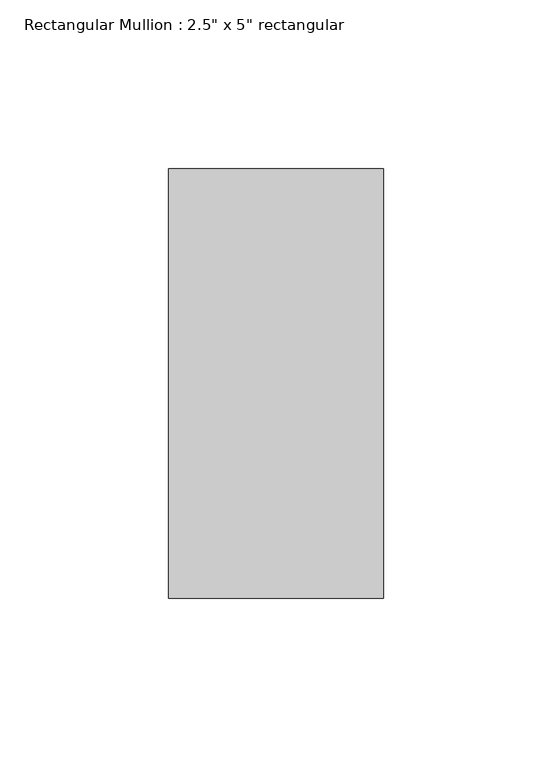
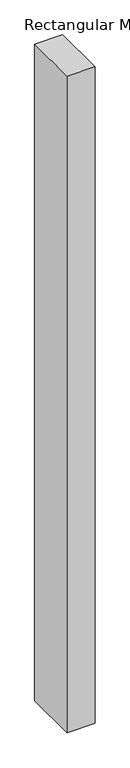
"""IFC4 building model written with IfcOpenShell, lengths in millimetres: member geometry."""

from ifc_helpers import new_model, si_unit, frame, origin, place, context, project, spatial, polyline, outline, extrude, source, transform, mapped, element, save


def member_ef177d9f(model_context):
    return source(origin(), model_context, "Body", "SweptSolid", [
        extrude(outline(polyline([(31.75, 63.5), (31.75, -63.5), (-31.75, -63.5), (-31.75, 63.5), (31.75, 63.5)])), frame((0.0, 0.0, -1576.4289848), z_axis=(0.0, 0.0, 1.0), x_axis=(1.0, 0.0, 0.0)), (0.0, 0.0, 1.0), 1576.4289848),
    ])


if __name__ == "__main__":
    model = new_model("IFC4")
    model_context = context("Model", 3, world=origin())
    ifc_project = project(units=[si_unit("LENGTHUNIT", "METRE", prefix="MILLI")], contexts=[model_context])
    site = spatial("IfcSite", under=ifc_project)
    building = spatial("IfcBuilding", under=site)
    placement = place(None, origin())
    member_shape = member_ef177d9f(model_context)
    element("IfcMember", 1, ObjectType="Rectangular Mullion : 2.5\" x 5\" rectangular", at=placement, inside=building, context=model_context, shape_type="MappedRepresentation", body=[
        mapped(member_shape, transform((0.0, 0.0, 0.0), x_axis=(1.0, 0.0, 0.0), y_axis=(0.0, 1.0, 0.0), z_axis=(0.0, 0.0, 1.0))),
    ])
    save(model, "model.ifc")

# Revit data of these elements
# Type "Rectangular Mullion : 2.5\" x 5\" rectangular"
#   built-in parameter 1007304 = 0.416667 (stored number, unit not read)
#   built-in parameter 1007301 = 0.104167 (stored number, unit not read)
#   built-in parameter 1007300 = 0.104167 (stored number, unit not read)
# Element 1 (IfcMember, "Rectangular Mullion : 2.5\" x 5\" rectangular")
#   Materials on its faces: "Aluminum"
# Materials
#   "Aluminum": class "Metal", colour RGB 247 247 247, transparency 0, Description = "Aluminum 6061", Cost = 0
